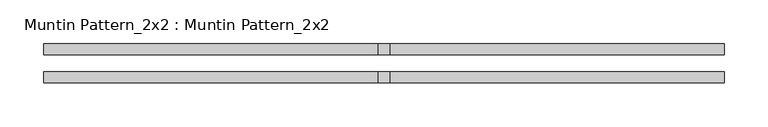
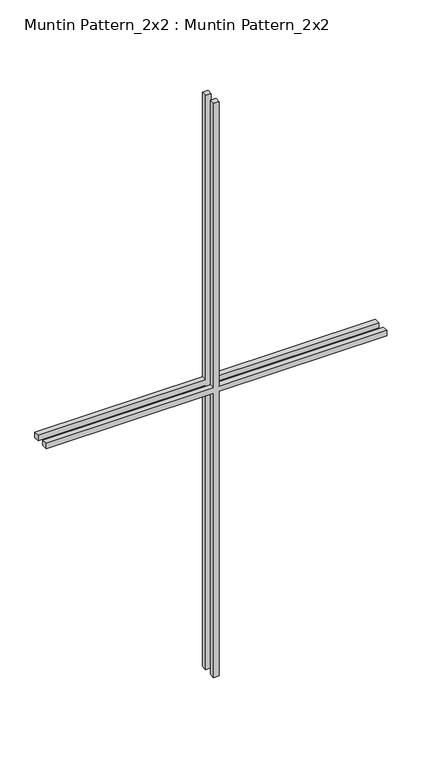
"""IFC4 building model written with IfcOpenShell, lengths in millimetres: proxy geometry, Muntin Pattern_2x2 : Muntin Pattern_2x2."""

from ifc_helpers import new_model, si_unit, frame, origin, place, context, project, spatial, polyline, outline, extrude, source, transform, mapped, element, save


def muntin_pattern_2x2_muntin_pattern_2x2_e751b040(model_context):
    return source(origin(), model_context, "Body", "SweptSolid", [
        extrude(outline(polyline([(698.5, -6.35), (698.5, -388.9375), (685.8, -388.9375), (685.8, -6.35), (0.0, -6.35), (0.0, 6.35), (685.8, 6.35), (685.8, 388.9375), (698.5, 388.9375), (698.5, 6.35), (1384.3, 6.35), (1384.3, -6.35), (698.5, -6.35)])), frame((0.0, 9.525, 0.0), z_axis=(0.0, 1.0, 0.0), x_axis=(0.0, 0.0, 1.0)), (0.0, 0.0, 1.0), 12.7),
        extrude(outline(polyline([(698.5, -6.35), (698.5, -388.9375), (685.8, -388.9375), (685.8, -6.35), (0.0, -6.35), (0.0, 6.35), (685.8, 6.35), (685.8, 388.9375), (698.5, 388.9375), (698.5, 6.35), (1384.3, 6.35), (1384.3, -6.35), (698.5, -6.35)])), frame((0.0, -22.225, 0.0), z_axis=(0.0, 1.0, 0.0), x_axis=(0.0, 0.0, 1.0)), (0.0, 0.0, 1.0), 12.7),
    ])


if __name__ == "__main__":
    model = new_model("IFC4")
    model_context = context("Model", 3, world=origin())
    ifc_project = project(units=[si_unit("LENGTHUNIT", "METRE", prefix="MILLI")], contexts=[model_context])
    site = spatial("IfcSite", under=ifc_project)
    building = spatial("IfcBuilding", under=site)
    placement = place(None, origin())
    muntin_pattern_2x2_muntin_pattern_2x2_shape = muntin_pattern_2x2_muntin_pattern_2x2_e751b040(model_context)
    element("IfcBuildingElementProxy", 1, Name="Muntin Pattern_2x2 : Muntin Pattern_2x2", ObjectType="Muntin Pattern_2x2 : Muntin Pattern_2x2", at=placement, inside=building, context=model_context, shape_type="MappedRepresentation", body=[
        mapped(muntin_pattern_2x2_muntin_pattern_2x2_shape, transform((0.0, 0.0, 0.0), x_axis=(1.0, 0.0, 0.0), y_axis=(0.0, 1.0, 0.0), z_axis=(0.0, 0.0, 1.0))),
    ])
    save(model, "model.ifc")

# Revit data of these elements
# Type "Muntin Pattern_2x2 : Muntin Pattern_2x2"
#   Width [instance default] = 4' - 0"
#   Thickness = 0' - 0 1/2"
#   Height [instance default] = 4' - 0"
#   Distance = 0' - 0 3/4"
#   Interior Material [instance default] = none
#   Exterior Material [instance default] = none
#   Default Elevation = 0
# Element 1 (IfcBuildingElementProxy, "Muntin Pattern_2x2 : Muntin Pattern_2x2")
#   Width = 2' - 6 5/8"
#   Height = 4' - 6 1/2"
#   Interior Material = Wood - Stained
#   Exterior Material = Clad - White
#   Materials on its faces: "Clad - White", "Wood - Stained"
# Materials
#   "Clad - White": class "Wood", colour RGB 242 242 238, transparency 0, Cost = 0
#   "Wood - Stained": class "Wood", colour RGB 224 178 126, transparency 0, Cost = 0
